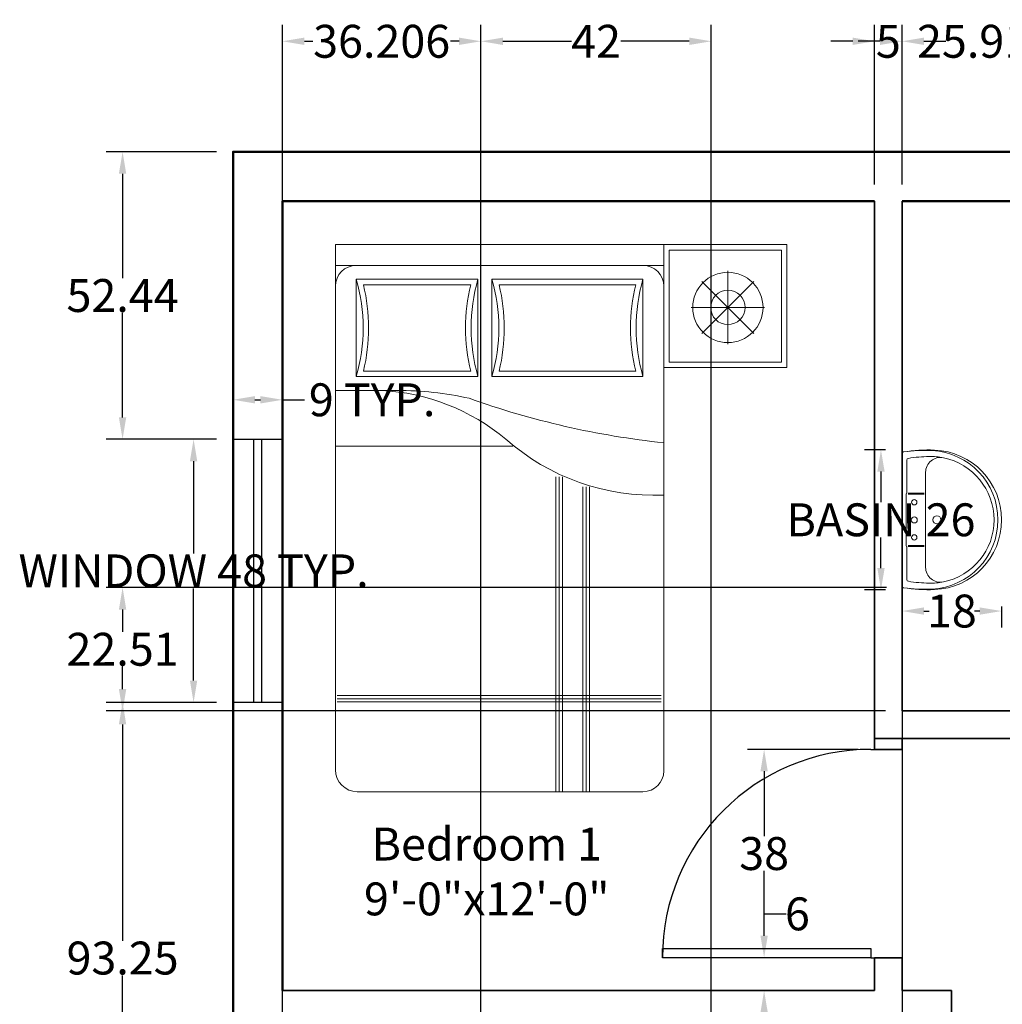
# Model space of a CAD drawing. Units: inches. Extents: x 89 to 490, y -59 to 378.
# Tile 19 of 20: x 89 to 268, y 198 to 378. Entities that reach past the tile are written whole.
import ezdxf

# ---------------------------------------------------------------- set-up
doc = ezdxf.new("R2010")
doc.units = ezdxf.units.IN
doc.header["$MEASUREMENT"] = 0
for name, color, linetype, lineweight in [('A-ANNO-DIMS', 2, 'Continuous', 18), ('A-AREA-IDEN', 7, 'Continuous', 18), ('Beds', 64, 'Continuous', 18), ('Doors', 34, 'Continuous', 25), ('Inner Walls', 31, 'Continuous', 35), ('Outer Walls', 12, 'Continuous', 50), ('Sink', 21, 'Continuous', 18), ('Windows', 171, 'Continuous', 25)]:
    doc.layers.add(name, color=color, linetype=linetype, lineweight=lineweight)
doc.styles.get("Standard").update_dxf_attribs({"font": 'arial.ttf'})
doc.dimstyles.get("Standard").update_dxf_attribs({"dimtxt": 6, "dimasz": 4, "dimexe": 3, "dimexo": 3, "dimgap": 0.09, "dimtad": 0, "dimtih": 1, "dimtoh": 1, "dimdec": 1, "dimzin": 0, "dimdsep": 46, "dimlunit": 3, "dimtxsty": 'Standard', "dimcen": 0.09, "dimadec": 0, "dimazin": 0, "dimtfac": 1, "dimtdec": 1, "dimtofl": 0, "dimtmove": 0, "dimatfit": 3, "dimfxl": 1, "dimtolj": 1, "dimtzin": 0, "dimarcsym": 0})

# ---------------------------------------------------------------- blocks, each defined once
blk = doc.blocks.new('*U6')
for p, q in [((0, 0), (0, -6)), ((40, 0), (40, -6))]:
    blk.add_line(p, q)
blk.add_lwpolyline([(0, 0), (0, 40), (1.75, 40), (1.75, 0)], close=True)
blk.add_arc((0, 0), 40, 0, 90)
blk = doc.blocks.new('A$C216962CD')
at = {"linetype": 'ByBlock'}
for p, q in [((0, 1.5502), (0, 2.0002)), ((0, 2.0002), (0.45, 2.0002)), ((0.45, 1.924), (0.45, 2.0002)), ((0.45, 2.0002), (0.45, 1.5502)), ((0.45, 2.0002), (1.6506, 2.0002)), ((1.6506, 2.0002), (1.6506, 1.5502)), ((0.45, 1.924), (1.6506, 1.924)), ((0.5262, 1.8732), (0.5262, 1.5176)), ((1.0785, 1.8732), (0.5262, 1.8732)), ((1.0785, 1.5176), (1.0785, 1.8732)), ((1.1293, 1.8732), (1.1293, 1.5176)), ((1.5744, 1.8732), (1.1293, 1.8732)), ((1.5744, 1.5176), (1.5744, 1.8732)), ((0.45, 0.0762), (0.45, 1.8478)), ((1.6506, 1.8478), (1.6506, 0.08)), ((0.45, 1.5502), (0, 1.5502)), ((0.5262, 1.5176), (1.0785, 1.5176)), ((1.1293, 1.5176), (1.5744, 1.5176)), ((1.4247, 1.4668), (1.6506, 1.4668)), ((1.0023, 1.2636), (1.6506, 1.2636)), ((1.5706, 0), (0.5262, 0))]:
    blk.add_line(p, q, dxfattribs=at)
for p, q in [((0.02, 1.5702), (0.02, 1.9802)), ((0.02, 1.9802), (0.43, 1.9802)), ((0.43, 1.9802), (0.43, 1.5702)), ((0.216, 1.7702), (0.216, 1.9046)), ((0.216, 1.7702), (0.121, 1.8652)), ((0.216, 1.7702), (0.3111, 1.8652)), ((1.0524, 1.8532), (0.5523, 1.8532)), ((1.5483, 1.8532), (1.1554, 1.8532)), ((0.216, 1.7702), (0.0817, 1.7702)), ((0.216, 1.7702), (0.121, 1.6752)), ((0.216, 1.7702), (0.216, 1.6358)), ((0.216, 1.7702), (0.3504, 1.7702)), ((0.216, 1.7702), (0.3111, 1.6752)), ((0.43, 1.5702), (0.02, 1.5702)), ((0.5523, 1.5376), (1.0524, 1.5376)), ((1.1554, 1.5376), (1.5483, 1.5376)), ((0.8202, 1.1507), (0.8202, 0)), ((0.8322, 1.1507), (0.8322, 0)), ((0.8442, 1.1507), (0.8442, 0)), ((0.722, 1.1146), (0.722, 0)), ((0.734, 1.1146), (0.734, 0)), ((0.746, 1.1146), (0.746, 0)), ((0.4599, 0.3521), (1.6437, 0.3521)), ((0.4599, 0.3401), (1.6437, 0.3401)), ((0.4599, 0.3281), (1.6437, 0.3281))]:
    blk.add_line(p, q)
for radius in [0.1285, 0.0628]:
    blk.add_circle((0.216, 1.7702), radius)
for centre, radius, start, end in [((0.5262, 1.8478), 0.0762, 90, 180), ((1.5744, 1.8478), 0.0762, 0, 90), ((-0.0834, 1.6954), 0.635, 343.7398, 16.2602), ((1.6881, 1.6954), 0.635, 163.7398, 196.2602), ((0.5197, 1.6954), 0.635, 343.7398, 16.2602), ((2.184, 1.6954), 0.635, 163.7398, 196.2602), ((1.5209, 0.6982), 0.7696, 92.9261, 129.8555), ((1.4243, 0.2475), 1.2193, 89.9814, 102.4667), ((0.1309, 4.3115), 3.0525, 275.9977, 289.7225), ((0.4856, 1.9017), 0.8181, 267.5082, 311.5038), ((0.5262, 0.0762), 0.0762, 180, 270), ((1.5706, 0.08), 0.08, 270, 0)]:
    blk.add_arc(centre, radius, start, end, dxfattribs=at)
for centre, start, end in [((-0.0834, 1.6954), 346.0594, 13.9406), ((1.6881, 1.6954), 166.0594, 193.9406), ((0.5197, 1.6954), 346.0594, 13.9406), ((2.184, 1.6954), 166.0594, 193.9406)]:
    blk.add_arc(centre, 0.655, start, end)
blk = doc.blocks.new('B2')
at = {"color": 0}
for p, q in [((-342.1, -28), (-155.1, -28)), ((-153.6, -35.9), (-153.6, -126.6)), ((-147.1, -24), (-0.5, -24)), ((-147.1, -35.9), (-147.1, -126.6)), ((147.1, -24), (-0.5, -24)), ((147.1, -35.9), (147.1, -126.6)), ((153.6, -35.9), (153.6, -126.6)), ((342.1, -28), (155.1, -28)), ((-0.5, -135), (-272, -135)), ((-0.5, -135), (272.1, -135))]:
    blk.add_line(p, q, dxfattribs=at)
blk.add_lwpolyline([(0, -570, -0.403574), (-399.2, -186.1, -0.04955), (-388.9, -8.4, -0.368901), (-379, 0), (0, 0), (379.1, 0, -0.368901), (388.9, -8.4, -0.04955), (399.3, -186.1, -0.40261)], format="xyb", close=True, dxfattribs=at)
for centre in [(-100.5, -70), (100.6, -70)]:
    blk.add_circle(centre, 15, dxfattribs=at)
for centre, radius, start, end in [((502.9, -129.4), 900, 172.2728, 182.7318), ((437.5, -165.7), 800, 170.697, 179.2737), ((-342.1, -38), 10, 90, 170.697), ((-155.1, -24), 4, 270, 323.1301), ((-147.1, -30), 6, 90, 143.1301), ((-0.5, -70), 17.5, 90, 270), ((-0.5, -70), 17.5, 270, 90), ((147.1, -30), 6, 36.8699, 90), ((155.1, -24), 4, 216.8699, 270), ((342.1, -38), 10, 9.303, 90), ((-437.5, -165.7), 800, 0.7263, 9.303), ((-502.9, -129.4), 900, 357.2682, 7.7272), ((-0.5, -165), 362, 178.5068, 191.4525), ((-272, -220), 85, 90, 191.4525), ((272.1, -220), 85, 348.5475, 90), ((0.6, -165), 362, 348.5475, 1.4932), ((-0.5, -153), 396, 182.7996, 270.0771), ((0, -200), 23, 90, 270), ((-0.4, -152), 397, 270.055, 357.0633), ((0, -200), 23, 270, 90), ((-0.5, -165), 362, 191.4525, 270.0843), ((-0.4, -163.8), 363.2, 270.0645, 348.3933)]:
    blk.add_arc(centre, radius, start, end, dxfattribs=at)
blk = doc.blocks.new('WIN-48x9')
for p, q in [((3.8, 0), (3.8, 48)), ((5.2, 48), (5.2, 0))]:
    blk.add_line(p, q)
blk.add_lwpolyline([(9, 0), (0, 0), (0, 48), (9, 48)], close=True)
blk = doc.blocks.new('*D22')
at = {"layer": 'A-ANNO-DIMS', "color": 0, "lineweight": -2, "transparency": 16777216}
for p, q in [((246.44, 299.4), (242.6, 299.4)), ((245.6, 295.4), (245.6, 289.8)), ((245.6, 277.81), (245.6, 283.41)), ((246.44, 273.81), (242.6, 273.81))]:
    blk.add_line(p, q, dxfattribs=at)
at = {"layer": 'A-ANNO-DIMS', "color": 0, "transparency": 16777216}
for points in [[(244.94, 295.4), (246.27, 295.4), (245.6, 299.4)], [(244.94, 277.81), (246.27, 277.81), (245.6, 273.81)]]:
    blk.add_solid(points, dxfattribs=at)
at = {"layer": 'Defpoints', "color": 0, "transparency": 16777216}
for p in [(245.6, 299.4), (249.44, 299.4), (249.44, 273.81)]:
    blk.add_point(p, dxfattribs=at)
at = {"layer": 'A-ANNO-DIMS', "color": 0, "transparency": 16777216, "insert": (245.6, 286.61), "char_height": 6, "attachment_point": 5}
blk.add_mtext('\\A1;BASIN 26', dxfattribs=at)
blk = doc.blocks.new('*D23')
at = {"layer": 'A-ANNO-DIMS', "color": 0, "lineweight": -2, "transparency": 16777216}
for p, q in [((249.44, 270.81), (249.44, 266.97)), ((253.44, 269.97), (254.41, 269.97)), ((263.61, 269.97), (262.64, 269.97)), ((267.61, 270.81), (267.61, 266.97))]:
    blk.add_line(p, q, dxfattribs=at)
at = {"layer": 'A-ANNO-DIMS', "color": 0, "transparency": 16777216}
for points in [[(253.44, 270.64), (253.44, 269.3), (249.44, 269.97)], [(263.61, 270.64), (263.61, 269.3), (267.61, 269.97)]]:
    blk.add_solid(points, dxfattribs=at)
at = {"layer": 'Defpoints', "color": 0, "transparency": 16777216}
for p in [(249.44, 273.81), (267.61, 273.81), (249.44, 269.97)]:
    blk.add_point(p, dxfattribs=at)
at = {"layer": 'A-ANNO-DIMS', "color": 0, "transparency": 16777216, "insert": (258.53, 269.97), "char_height": 6, "attachment_point": 5}
blk.add_mtext('\\A1;18', dxfattribs=at)
blk = doc.blocks.new('*D32')
at = {"layer": 'A-ANNO-DIMS', "color": 0, "lineweight": -2, "transparency": 16777216}
for p, q in [((124.44, 301.3), (117.24, 301.3)), ((120.24, 297.3), (120.24, 280.49)), ((120.24, 257.3), (120.24, 274.11)), ((124.44, 253.3), (117.24, 253.3))]:
    blk.add_line(p, q, dxfattribs=at)
at = {"layer": 'A-ANNO-DIMS', "color": 0, "transparency": 16777216}
for points in [[(119.57, 297.3), (120.91, 297.3), (120.24, 301.3)], [(119.57, 257.3), (120.91, 257.3), (120.24, 253.3)]]:
    blk.add_solid(points, dxfattribs=at)
at = {"layer": 'Defpoints', "color": 0, "transparency": 16777216}
for p in [(120.24, 301.3), (127.44, 301.3), (127.44, 253.3)]:
    blk.add_point(p, dxfattribs=at)
at = {"layer": 'A-ANNO-DIMS', "color": 0, "transparency": 16777216, "insert": (120.24, 277.3), "char_height": 6, "attachment_point": 5}
blk.add_mtext('\\A1;WINDOW 48 TYP.', dxfattribs=at)
blk = doc.blocks.new('*D33')
at = {"layer": 'A-ANNO-DIMS', "color": 0, "lineweight": -2, "transparency": 16777216}
for p, q in [((127.44, 304.3), (127.44, 311.5)), ((136.44, 304.3), (136.44, 311.5)), ((131.44, 308.5), (132.44, 308.5)), ((136.44, 308.5), (140.44, 308.5))]:
    blk.add_line(p, q, dxfattribs=at)
at = {"layer": 'A-ANNO-DIMS', "color": 0, "transparency": 16777216}
for points in [[(131.44, 309.17), (131.44, 307.83), (127.44, 308.5)], [(132.44, 309.17), (132.44, 307.83), (136.44, 308.5)]]:
    blk.add_solid(points, dxfattribs=at)
at = {"layer": 'Defpoints', "color": 0, "transparency": 16777216}
for p in [(136.44, 308.5), (127.44, 301.3), (136.44, 301.3)]:
    blk.add_point(p, dxfattribs=at)
at = {"layer": 'A-ANNO-DIMS', "color": 0, "transparency": 16777216, "insert": (152.8, 308.5), "char_height": 6, "attachment_point": 5}
blk.add_mtext('\\A1;9 TYP.', dxfattribs=at)
blk = doc.blocks.new('*D51')
at = {"layer": 'A-ANNO-DIMS', "color": 0, "lineweight": -2, "transparency": 16777216}
for p, q in [((124.44, 353.74), (104.29, 353.74)), ((107.29, 349.74), (107.29, 330.67)), ((107.29, 305.3), (107.29, 324.37)), ((124.44, 301.3), (104.29, 301.3))]:
    blk.add_line(p, q, dxfattribs=at)
at = {"layer": 'A-ANNO-DIMS', "color": 0, "transparency": 16777216}
for points in [[(106.62, 349.74), (107.96, 349.74), (107.29, 353.74)], [(106.62, 305.3), (107.96, 305.3), (107.29, 301.3)]]:
    blk.add_solid(points, dxfattribs=at)
at = {"layer": 'Defpoints', "color": 0, "transparency": 16777216}
for p in [(127.44, 353.74), (107.29, 301.3), (127.44, 301.3)]:
    blk.add_point(p, dxfattribs=at)
at = {"layer": 'A-ANNO-DIMS', "color": 0, "transparency": 16777216, "insert": (107.29, 327.52), "char_height": 6, "attachment_point": 5}
blk.add_mtext('\\A1;52.44', dxfattribs=at)
blk = doc.blocks.new('*D52')
at = {"layer": 'A-ANNO-DIMS', "color": 0, "lineweight": -2, "transparency": 16777216}
for p, q in [((124.44, 253.3), (104.29, 253.3)), ((107.29, 249.3), (107.29, 209.83)), ((107.29, 164.06), (107.29, 203.52)), ((124.44, 160.06), (104.29, 160.06))]:
    blk.add_line(p, q, dxfattribs=at)
at = {"layer": 'A-ANNO-DIMS', "color": 0, "transparency": 16777216}
for points in [[(106.62, 249.3), (107.96, 249.3), (107.29, 253.3)], [(106.62, 164.06), (107.96, 164.06), (107.29, 160.06)]]:
    blk.add_solid(points, dxfattribs=at)
at = {"layer": 'Defpoints', "color": 0, "transparency": 16777216}
for p in [(127.44, 253.3), (107.29, 160.06), (127.44, 160.06)]:
    blk.add_point(p, dxfattribs=at)
at = {"layer": 'A-ANNO-DIMS', "color": 0, "transparency": 16777216, "insert": (107.29, 206.68), "char_height": 6, "attachment_point": 5}
blk.add_mtext('\\A1;93.25', dxfattribs=at)
blk = doc.blocks.new('*D53')
at = {"layer": 'A-ANNO-DIMS', "color": 0, "lineweight": -2, "transparency": 16777216}
for p, q in [((249.44, 347.74), (249.44, 376.89)), ((275.35, 356.74), (275.35, 376.89)), ((245.44, 373.89), (241.44, 373.89)), ((279.35, 373.89), (283.35, 373.89))]:
    blk.add_line(p, q, dxfattribs=at)
at = {"layer": 'A-ANNO-DIMS', "color": 0, "transparency": 16777216}
for points in [[(245.44, 374.56), (245.44, 373.22), (249.44, 373.89)], [(279.35, 374.56), (279.35, 373.22), (275.35, 373.89)]]:
    blk.add_solid(points, dxfattribs=at)
at = {"layer": 'Defpoints', "color": 0, "transparency": 16777216}
for p in [(275.35, 373.89), (275.35, 353.74), (249.44, 344.74)]:
    blk.add_point(p, dxfattribs=at)
at = {"layer": 'A-ANNO-DIMS', "color": 0, "transparency": 16777216, "insert": (262.4, 373.89), "char_height": 6, "attachment_point": 5}
blk.add_mtext('\\A1;25.91', dxfattribs=at)
blk = doc.blocks.new('*D54')
at = {"layer": 'A-ANNO-DIMS', "color": 0, "lineweight": -2, "transparency": 16777216}
for p, q in [((244.44, 347.74), (244.44, 376.89)), ((249.44, 347.74), (249.44, 376.89)), ((240.44, 373.89), (236.44, 373.89)), ((253.44, 373.89), (257.44, 373.89))]:
    blk.add_line(p, q, dxfattribs=at)
at = {"layer": 'A-ANNO-DIMS', "color": 0, "transparency": 16777216}
for points in [[(240.44, 374.56), (240.44, 373.22), (244.44, 373.89)], [(253.44, 374.56), (253.44, 373.22), (249.44, 373.89)]]:
    blk.add_solid(points, dxfattribs=at)
at = {"layer": 'Defpoints', "color": 0, "transparency": 16777216}
for p in [(249.44, 373.89), (244.44, 344.74), (249.44, 344.74)]:
    blk.add_point(p, dxfattribs=at)
at = {"layer": 'A-ANNO-DIMS', "color": 0, "transparency": 16777216, "insert": (246.94, 373.89), "char_height": 6, "attachment_point": 5}
blk.add_mtext('\\A1;5', dxfattribs=at)
blk = doc.blocks.new('*D57')
at = {"layer": 'A-ANNO-DIMS', "color": 0, "lineweight": -2, "transparency": 16777216}
for p, q in [((172.65, 75.74), (172.65, 376.89)), ((214.65, 75.74), (214.65, 376.89)), ((176.65, 373.89), (189.17, 373.89)), ((210.65, 373.89), (198.13, 373.89))]:
    blk.add_line(p, q, dxfattribs=at)
at = {"layer": 'A-ANNO-DIMS', "color": 0, "transparency": 16777216}
for points in [[(176.65, 374.56), (176.65, 373.22), (172.65, 373.89)], [(210.65, 374.56), (210.65, 373.22), (214.65, 373.89)]]:
    blk.add_solid(points, dxfattribs=at)
at = {"layer": 'Defpoints', "color": 0, "transparency": 16777216}
for p in [(214.65, 373.89), (172.65, 72.74), (214.65, 72.74)]:
    blk.add_point(p, dxfattribs=at)
at = {"layer": 'A-ANNO-DIMS', "color": 0, "transparency": 16777216, "insert": (193.65, 373.89), "char_height": 6, "attachment_point": 5}
blk.add_mtext('\\A1;42', dxfattribs=at)
blk = doc.blocks.new('*D58')
at = {"layer": 'A-ANNO-DIMS', "color": 0, "lineweight": -2, "transparency": 16777216}
for p, q in [((136.44, 75.74), (136.44, 376.89)), ((172.65, 75.74), (172.65, 376.89)), ((140.44, 373.89), (142, 373.89)), ((168.65, 373.89), (167.08, 373.89))]:
    blk.add_line(p, q, dxfattribs=at)
at = {"layer": 'A-ANNO-DIMS', "color": 0, "transparency": 16777216}
for points in [[(140.44, 374.56), (140.44, 373.22), (136.44, 373.89)], [(168.65, 374.56), (168.65, 373.22), (172.65, 373.89)]]:
    blk.add_solid(points, dxfattribs=at)
at = {"layer": 'Defpoints', "color": 0, "transparency": 16777216}
for p in [(172.65, 373.89), (136.44, 72.74), (172.65, 72.74)]:
    blk.add_point(p, dxfattribs=at)
at = {"layer": 'A-ANNO-DIMS', "color": 0, "transparency": 16777216, "insert": (154.54, 373.89), "char_height": 6, "attachment_point": 5}
blk.add_mtext('\\A1;36.206', dxfattribs=at)
blk = doc.blocks.new('*D59')
at = {"layer": 'A-ANNO-DIMS', "color": 0, "lineweight": -2, "transparency": 16777216}
for p, q in [((241.44, 244.74), (221.29, 244.74)), ((224.29, 240.74), (224.29, 228.9)), ((224.29, 210.74), (224.29, 222.59)), ((241.44, 206.74), (221.29, 206.74))]:
    blk.add_line(p, q, dxfattribs=at)
at = {"layer": 'A-ANNO-DIMS', "color": 0, "transparency": 16777216}
for points in [[(223.62, 240.74), (224.96, 240.74), (224.29, 244.74)], [(223.62, 210.74), (224.96, 210.74), (224.29, 206.74)]]:
    blk.add_solid(points, dxfattribs=at)
at = {"layer": 'Defpoints', "color": 0, "transparency": 16777216}
for p in [(224.29, 244.74), (244.44, 244.74), (244.44, 206.74)]:
    blk.add_point(p, dxfattribs=at)
at = {"layer": 'A-ANNO-DIMS', "color": 0, "transparency": 16777216, "insert": (224.29, 225.74), "char_height": 6, "attachment_point": 5}
blk.add_mtext('\\A1;38', dxfattribs=at)
blk = doc.blocks.new('*D60')
at = {"layer": 'A-ANNO-DIMS', "color": 0, "lineweight": -2, "transparency": 16777216}
for p, q in [((224.29, 210.74), (224.29, 214.74)), ((224.29, 214.74), (228.29, 214.74)), ((241.44, 206.74), (221.29, 206.74)), ((241.44, 200.74), (221.29, 200.74)), ((224.29, 196.74), (224.29, 192.74))]:
    blk.add_line(p, q, dxfattribs=at)
at = {"layer": 'A-ANNO-DIMS', "color": 0, "transparency": 16777216}
for points in [[(223.62, 210.74), (224.96, 210.74), (224.29, 206.74)], [(223.62, 196.74), (224.96, 196.74), (224.29, 200.74)]]:
    blk.add_solid(points, dxfattribs=at)
at = {"layer": 'Defpoints', "color": 0, "transparency": 16777216}
for p in [(224.29, 206.74), (244.44, 206.74), (244.44, 200.74)]:
    blk.add_point(p, dxfattribs=at)
at = {"layer": 'A-ANNO-DIMS', "color": 0, "transparency": 16777216, "insert": (230.36, 214.74), "char_height": 6, "attachment_point": 5}
blk.add_mtext('\\A1;6', dxfattribs=at)
blk = doc.blocks.new('*D73')
at = {"layer": 'A-ANNO-DIMS', "color": 0, "lineweight": -2, "transparency": 16777216}
for p, q in [((246.6, 274.25), (104.29, 274.25)), ((107.29, 270.25), (107.29, 266.15)), ((107.29, 255.74), (107.29, 259.84)), ((246.44, 251.74), (104.29, 251.74))]:
    blk.add_line(p, q, dxfattribs=at)
at = {"layer": 'A-ANNO-DIMS', "color": 0, "transparency": 16777216}
for points in [[(106.62, 270.25), (107.96, 270.25), (107.29, 274.25)], [(106.62, 255.74), (107.96, 255.74), (107.29, 251.74)]]:
    blk.add_solid(points, dxfattribs=at)
at = {"layer": 'Defpoints', "color": 0, "transparency": 16777216}
for p in [(107.29, 274.25), (249.6, 274.25), (249.44, 251.74)]:
    blk.add_point(p, dxfattribs=at)
at = {"layer": 'A-ANNO-DIMS', "color": 0, "transparency": 16777216, "insert": (107.29, 263), "char_height": 6, "attachment_point": 5}
blk.add_mtext('\\A1;22.51', dxfattribs=at)
blk = doc.blocks.new('*D74')
at = {"layer": 'A-ANNO-DIMS', "color": 0, "lineweight": -2, "transparency": 16777216}
for p, q in [((249.44, 341.74), (249.44, -49.81)), ((277.75, 341.35), (277.75, -49.81)), ((253.44, -46.81), (253.91, -46.81)), ((273.75, -46.81), (273.28, -46.81))]:
    blk.add_line(p, q, dxfattribs=at)
at = {"layer": 'A-ANNO-DIMS', "color": 0, "transparency": 16777216}
for points in [[(253.44, -46.14), (253.44, -47.48), (249.44, -46.81)], [(273.75, -46.14), (273.75, -47.48), (277.75, -46.81)]]:
    blk.add_solid(points, dxfattribs=at)
at = {"layer": 'Defpoints', "color": 0, "transparency": 16777216}
for p in [(249.44, 344.74), (277.75, 344.35), (277.75, -46.81)]:
    blk.add_point(p, dxfattribs=at)
at = {"layer": 'A-ANNO-DIMS', "color": 0, "transparency": 16777216, "insert": (263.6, -46.81), "char_height": 6, "attachment_point": 5}
blk.add_mtext('\\A1;28.31', dxfattribs=at)

msp = doc.modelspace()

# ---------------------------------------------------------------- linework, layer by layer
at = {"layer": 'Inner Walls'}
for p, q in [((244.4414, 244.7413), (244.4414, 344.7413)), ((249.4414, 251.7413), (249.4414, 344.7413)), ((249.4414, 251.7413), (283.4414, 251.7413)), ((244.4414, 246.7413), (283.4414, 246.7413)), ((249.4414, 244.7413), (249.4414, 246.7413)), ((244.4414, 244.7413), (249.4414, 244.7413)), ((244.4414, 200.7413), (244.4414, 206.7413)), ((244.4414, 206.7413), (249.4414, 206.7413)), ((249.4414, 200.7413), (249.4414, 206.7413)), ((136.4414, 200.7413), (244.4414, 200.7413)), ((249.4414, 200.7413), (258.4414, 200.7413)), ((258.4414, 195.7413), (258.4414, 200.7413))]:
    msp.add_line(p, q, dxfattribs=at)
at = {"layer": 'Outer Walls'}
for p, q in [((136.4414, 344.7413), (244.4414, 344.7413)), ((136.4414, 200.7413), (136.4414, 344.7413)), ((249.4414, 344.7413), (325.4414, 344.7413))]:
    msp.add_line(p, q, dxfattribs=at)
msp.add_lwpolyline([(214.6478, 67.7413), (265.4414, 67.7413), (265.4414, 4.7413), (459.4414, 4.7413), (459.4414, 353.7413), (127.4414, 353.7413), (127.4414, 13.7413)], dxfattribs=at)

# ---------------------------------------------------------------- block references
at = {"layer": 'Beds', "xscale": -49.89604989604899, "yscale": 49.89604989604899, "zscale": 49.89604989604899}
msp.add_blockref('A$C216962CD', (228.4567, 237.014), dxfattribs=at)
at = {"layer": 'Doors', "xscale": 0.9500000000000021, "yscale": 0.9500000000000021, "zscale": 0.9500000000000021, "rotation": 90}
msp.add_blockref('*U6', (243.7414, 206.7413), dxfattribs=at)
at = {"layer": 'Sink', "xscale": 0.0318595969266409, "yscale": 0.0318595969266409, "zscale": 0.0318595969266409, "rotation": 90}
msp.add_blockref('B2', (249.4414, 286.6059), dxfattribs=at)
at = {"layer": 'Windows'}
msp.add_blockref('WIN-48x9', (127.441, 253.3003), dxfattribs=at)

# ---------------------------------------------------------------- texts
at = {"layer": 'A-AREA-IDEN', "insert": (150.5089, 230.4677), "char_height": 6, "attachment_point": 1}
msp.add_mtext_dynamic_manual_height_columns('\\pxqc;Bedroom 1\\P9\'-0"x12\'-0"', width=46.403971, gutter_width=1, heights=[0], dxfattribs=at)

# ---------------------------------------------------------------- dimensions: what is measured, and where the dimension line sits
at = {"layer": 'A-ANNO-DIMS'}
for base, p1, p2, override, picture, middle in [((172.6478, 373.8913), (136.4414, 72.7413), (172.6478, 72.7413), {"dimdec": 3, "dimlfac": 1, "dimrnd": 0, "dimzin": 0, "dimdsep": 46, "dimlunit": 2}, '*D58', (154.5446, 373.8913)), ((214.6478, 373.8913), (172.6478, 72.7413), (214.6478, 72.7413), {"dimdec": 0, "dimlfac": 1, "dimrnd": 0, "dimzin": 0, "dimdsep": 46, "dimlunit": 2}, '*D57', (193.6478, 373.8913)), ((249.4414, 373.8913), (244.4414, 344.7413), (249.4414, 344.7413), {"dimdec": 0, "dimlfac": 1, "dimrnd": 0, "dimzin": 0, "dimdsep": 46, "dimlunit": 2}, '*D54', (246.9414, 373.8913)), ((275.3499, 373.8913), (249.4414, 344.7413), (275.3499, 353.7413), {"dimdec": 2, "dimlfac": 1, "dimrnd": 0, "dimzin": 0, "dimdsep": 46, "dimlunit": 2}, '*D53', (262.3956, 373.8913)), ((277.7535, -46.8094), (249.4414, 344.7413), (277.7535, 344.3468), {"dimdec": 2, "dimlfac": 1, "dimrnd": 0, "dimzin": 0, "dimdsep": 46, "dimlunit": 2}, '*D74', (263.5974, -46.8094))]:
    dim = msp.add_linear_dim(base=base, p1=p1, p2=p2, dimstyle='Standard', override=override, dxfattribs=at)
    dim.commit()
    dim.dimension.update_dxf_attribs({"geometry": picture, "text_midpoint": middle})
for base, p1, p2, angle, override, picture, middle in [((107.2914, 301.3003), (127.4414, 353.7413), (127.4414, 301.3003), 90, {"dimdec": 2, "dimlfac": 1, "dimrnd": 0, "dimzin": 0, "dimdsep": 46, "dimlunit": 2}, '*D51', (107.2914, 327.5208)), ((107.2914, 274.2529), (249.4414, 251.7413), (249.6029, 274.2529), 90, {"dimdec": 2, "dimlfac": 1, "dimrnd": 0, "dimzin": 0, "dimdsep": 46, "dimlunit": 2}, '*D73', (107.2914, 262.9971)), ((249.4414, 269.9693), (267.6105, 273.8086), (249.4414, 273.8086), 180, {"dimdec": 0, "dimlfac": 1, "dimrnd": 0, "dimzin": 0, "dimdsep": 46, "dimlunit": 2}, '*D23', (258.5259, 269.9693)), ((107.2914, 160.055), (127.4414, 253.3003), (127.4414, 160.055), 90, {"dimdec": 2, "dimlfac": 1, "dimrnd": 0, "dimzin": 0, "dimdsep": 46, "dimlunit": 2}, '*D52', (107.2914, 206.6776)), ((224.2914, 244.7413), (244.4414, 206.7413), (244.4414, 244.7413), 90, {"dimdec": 0, "dimlfac": 1, "dimrnd": 0, "dimzin": 0, "dimdsep": 46, "dimlunit": 2}, '*D59', (224.2914, 225.7413)), ((224.2914, 206.7413), (244.4414, 200.7413), (244.4414, 206.7413), 90, {"dimdec": 0, "dimlfac": 1, "dimrnd": 0, "dimzin": 0, "dimdsep": 46, "dimlunit": 2}, '*D60', (230.3623, 214.7413))]:
    dim = msp.add_linear_dim(base=base, p1=p1, p2=p2, angle=angle, dimstyle='Standard', override=override, dxfattribs=at)
    dim.commit()
    dim.dimension.update_dxf_attribs({"geometry": picture, "text_midpoint": middle})
dim = msp.add_linear_dim(base=(136.4414, 308.5003), p1=(127.4414, 301.3003), p2=(136.4414, 301.3003), text='<> TYP.', dimstyle='Standard', override={"dimdec": 0, "dimlfac": 1, "dimrnd": 0, "dimzin": 0, "dimdsep": 46, "dimlunit": 2}, dxfattribs=at)
dim.commit()
dim.dimension.update_dxf_attribs({"geometry": '*D33', "text_midpoint": (152.8036, 308.5003)})
for base, p1, p2, text, picture, middle in [((120.2414, 301.3003), (127.4414, 253.3003), (127.4414, 301.3003), 'WINDOW <> TYP.', '*D32', (120.2414, 277.3003)), ((245.602, 299.4043), (249.4414, 273.8086), (249.4414, 299.4043), 'BASIN <>', '*D22', (245.602, 286.6065))]:
    dim = msp.add_linear_dim(base=base, p1=p1, p2=p2, angle=90, text=text, dimstyle='Standard', override={"dimdec": 0, "dimlfac": 1, "dimrnd": 0, "dimzin": 0, "dimdsep": 46, "dimlunit": 2}, dxfattribs=at)
    dim.commit()
    dim.dimension.update_dxf_attribs({"geometry": picture, "text_midpoint": middle})

doc.saveas('drawing.dxf')
